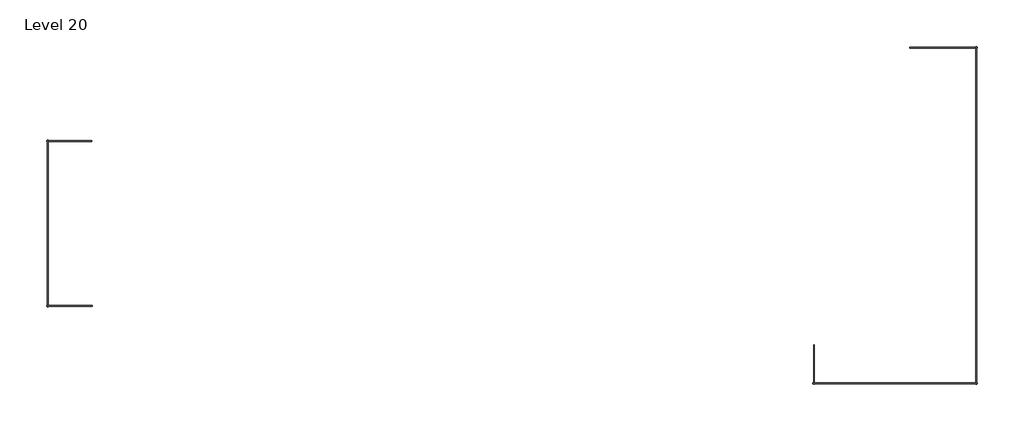
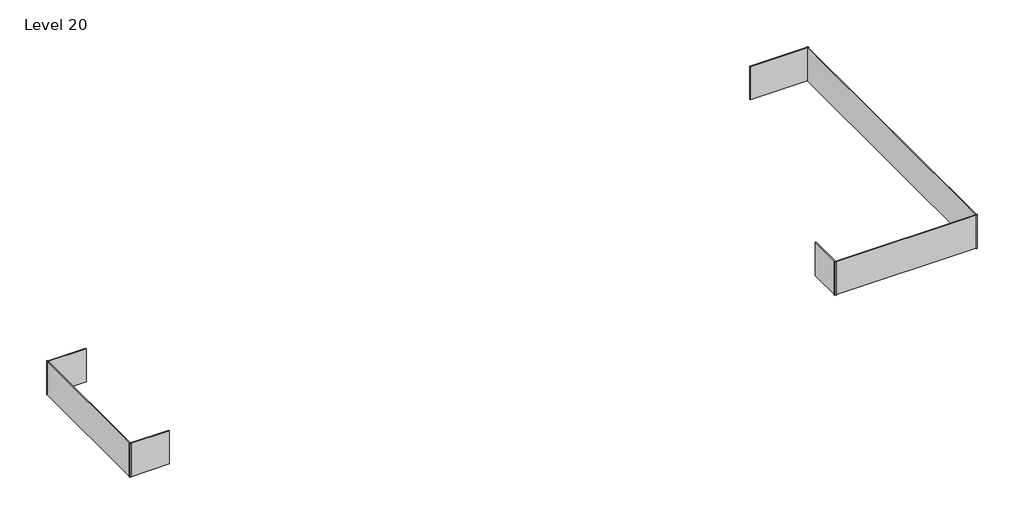
# One storey: 7 plates.
"""IFC4 building model written with IfcOpenShell, lengths in millimetres."""

from ifc_helpers import new_model, si_unit, origin, place, context, project, spatial, transform, mapped, element, save
from components import system_panel_glazed_246808bb, system_panel_glazed_a5f349e9, system_panel_glazed_67cddadf, system_panel_glazed_f6fb2dd6, system_panel_glazed_b1131520, system_panel_glazed_51f6397d, system_panel_glazed_7481726a

model = new_model("IFC4")

# Units and contexts
model_context = context("Model", 3, world=origin())
ifc_project = project(units=[si_unit("LENGTHUNIT", "METRE", prefix="MILLI")], contexts=[model_context])

# Site, building, storey
site = spatial("IfcSite", under=ifc_project)
building = spatial("IfcBuilding", under=site)
storey = spatial("IfcBuildingStorey", under=building, Name="Level 20", Elevation=32537.4)

# Plates
placement = place(None, origin())
system_panel_glazed_shape = system_panel_glazed_246808bb(model_context)
element("IfcPlate", 1, ObjectType="System Panel : Glazed", at=placement, inside=storey, context=model_context, shape_type="MappedRepresentation", body=[
    mapped(system_panel_glazed_shape, transform((-17311.9050371, -13712.8739591, 32537.4), x_axis=(1.0, 0.0, 0.0), y_axis=(0.0, 1.0, 0.0), z_axis=(0.0, 0.0, 1.0))),
])
system_panel_glazed_2_shape = system_panel_glazed_a5f349e9(model_context)
element("IfcPlate", 2, ObjectType="System Panel : Glazed", at=placement, inside=storey, context=model_context, shape_type="MappedRepresentation", body=[
    mapped(system_panel_glazed_2_shape, transform((-17997.7050371, -11201.4489591, 32537.4), x_axis=(0.0, -1.0, 0.0), y_axis=(1.0, 0.0, 0.0), z_axis=(0.0, 0.0, 1.0))),
])
system_panel_glazed_3_shape = system_panel_glazed_67cddadf(model_context)
element("IfcPlate", 3, ObjectType="System Panel : Glazed", at=placement, inside=storey, context=model_context, shape_type="MappedRepresentation", body=[
    mapped(system_panel_glazed_3_shape, transform((-17315.5277899, -8690.0239591, 32537.4), x_axis=(-1.0, 0.0, 0.0), y_axis=(0.0, -1.0, 0.0), z_axis=(0.0, 0.0, 1.0))),
])
system_panel_glazed_4_shape = system_panel_glazed_f6fb2dd6(model_context)
element("IfcPlate", 4, ObjectType="System Panel : Glazed", at=placement, inside=storey, context=model_context, shape_type="MappedRepresentation", body=[
    mapped(system_panel_glazed_4_shape, transform((5069.3964352, -15455.0778294, 32537.4), x_axis=(0.0, -1.0, 0.0), y_axis=(1.0, 0.0, 0.0), z_axis=(0.0, 0.0, 1.0))),
])
system_panel_glazed_5_shape = system_panel_glazed_b1131520(model_context)
element("IfcPlate", 5, ObjectType="System Panel : Glazed", at=placement, inside=storey, context=model_context, shape_type="MappedRepresentation", body=[
    mapped(system_panel_glazed_5_shape, transform((10022.3964352, -10959.2778294, 32537.4), x_axis=(0.0, 1.0, 0.0), y_axis=(-1.0, 0.0, 0.0), z_axis=(0.0, 0.0, 1.0))),
])
system_panel_glazed_6_shape = system_panel_glazed_51f6397d(model_context)
element("IfcPlate", 6, ObjectType="System Panel : Glazed", at=placement, inside=storey, context=model_context, shape_type="MappedRepresentation", body=[
    mapped(system_panel_glazed_6_shape, transform((7545.8964352, -16051.9778294, 32537.4), x_axis=(1.0, 0.0, 0.0), y_axis=(0.0, 1.0, 0.0), z_axis=(0.0, 0.0, 1.0))),
])
system_panel_glazed_7_shape = system_panel_glazed_7481726a(model_context)
element("IfcPlate", 7, ObjectType="System Panel : Glazed", at=placement, inside=storey, context=model_context, shape_type="MappedRepresentation", body=[
    mapped(system_panel_glazed_7_shape, transform((9006.3964352, -5866.5778294, 32537.4), x_axis=(-1.0, 0.0, 0.0), y_axis=(0.0, -1.0, 0.0), z_axis=(0.0, 0.0, 1.0))),
])

save(model, "model.ifc")

# Revit data of these elements
# Type "System Panel : Glazed"
#   Construction Type Id = "GSP4R"
#   Analytic Construction = "1/8 in Pilkington single glazing"
#   Visual Light Transmittance = 0.9
#   Solar Heat Gain Coefficient = 0.86
#   Heat Transfer Coefficient (U) = 1.18115 BTU/(h·ft²·°F)
# Elements 1, 2, 3, 4, 5, 6, 7 (IfcPlate, "System Panel : Glazed")
#   Phase Created = New Construction
#   Materials on its faces: "Glass"
# Materials
#   "Glass": class "Glass", colour RGB 0 128 192, transparency 0.75, Description = "Soda Lime Glass", Cost = 0
